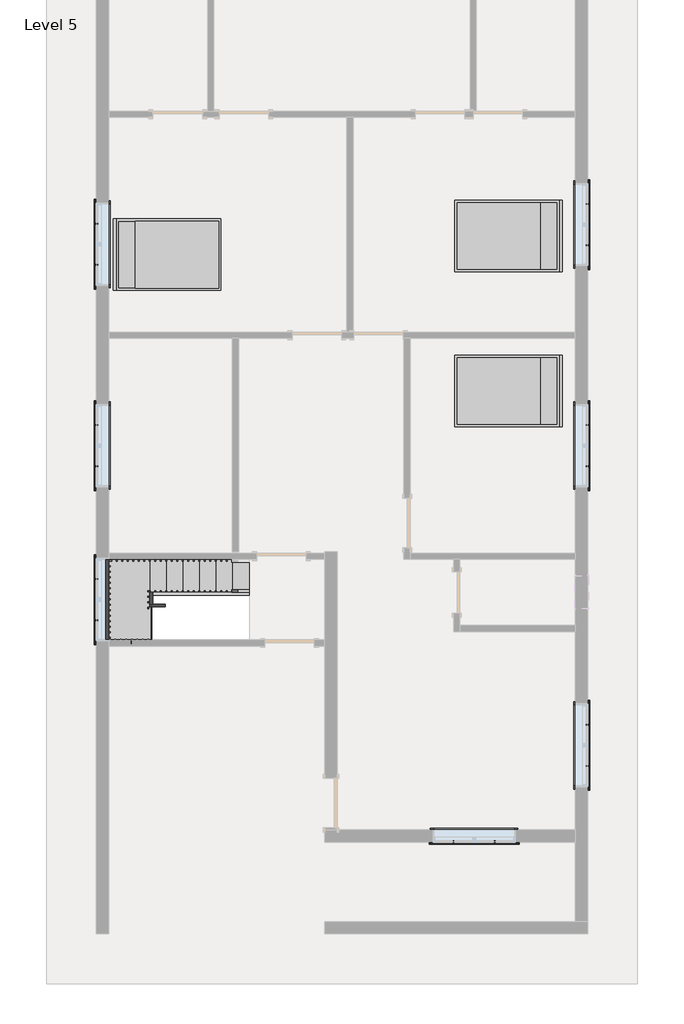
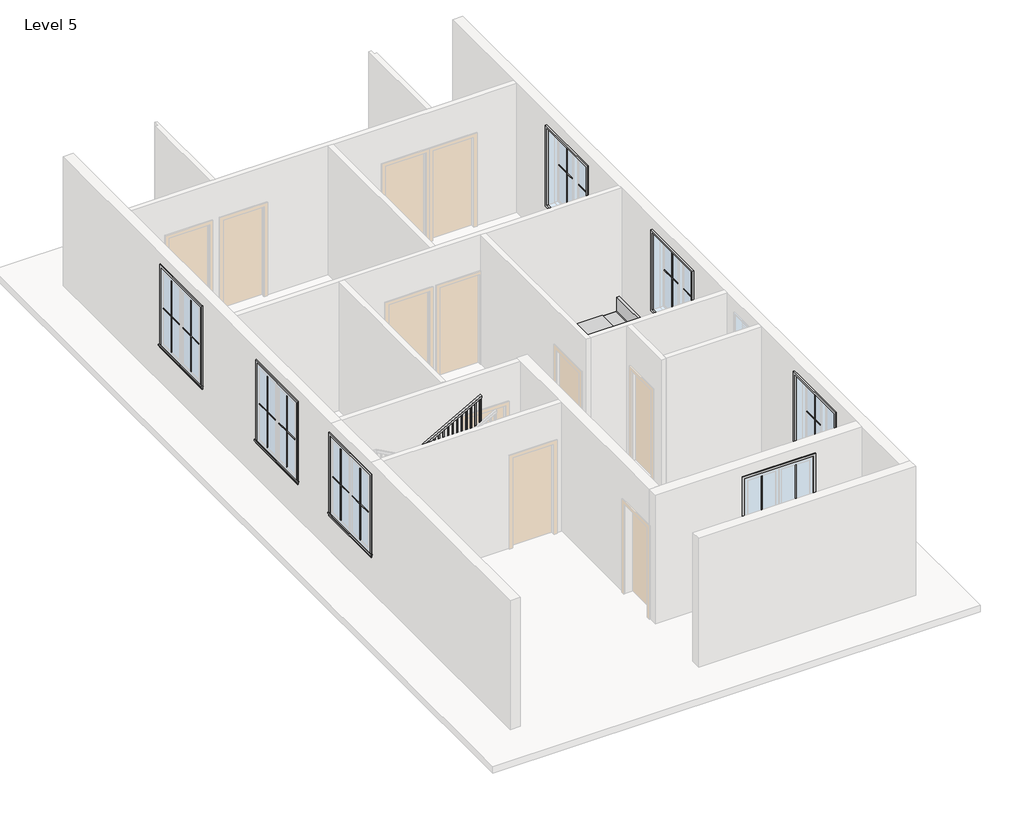
# One storey, part 3 of 3: 28 proxies, 6 members, 3 furniture elements, 1 railing, 1 stair flight.
"""IFC4 building model written with IfcOpenShell, lengths in millimetres."""

from ifc_helpers import new_model, si_unit, frame, origin, place, context, project, spatial, polyline, outline, extrude, faceted_brep, transform, mapped, element, save
from components import muntin_pattern_2x2_muntin_pattern_2x2_f6a80940, muntin_pattern_2x2_muntin_pattern_2x2_09b00a1c, trim_window_exterior_flat_with_sill_698ed857, trim_window_interior_flat_picture_frame_92551a5e, bed_17739_bed_17739_15c61121, stair_flight_98403923

model = new_model("IFC4")

# Units and contexts
model_context = context("Model", 3, world=origin())
ifc_project = project(units=[si_unit("LENGTHUNIT", "METRE", prefix="MILLI")], contexts=[model_context])

# Site, building, storey
site = spatial("IfcSite", under=ifc_project)
building = spatial("IfcBuilding", under=site)
storey = spatial("IfcBuildingStorey", under=building, Name="Level 5", Elevation=9601.2)

# Proxies
placement = place(None, origin())
muntin_pattern_2x2_muntin_pattern_2x2_shape = muntin_pattern_2x2_muntin_pattern_2x2_f6a80940(model_context)
element("IfcBuildingElementProxy", 1, Name="Muntin Pattern_2x2 : Muntin Pattern_2x2", ObjectType="Muntin Pattern_2x2 : Muntin Pattern_2x2", at=placement, inside=storey, context=model_context, shape_type="MappedRepresentation", body=[
    mapped(muntin_pattern_2x2_muntin_pattern_2x2_shape, transform((-5778.6870155, 3260.8309309, 10585.45), x_axis=(0.0, 1.0, 0.0), y_axis=(-1.0, 0.0, 0.0), z_axis=(0.0, 0.0, 1.0))),
])
element("IfcBuildingElementProxy", 2, Name="Muntin Pattern_2x2 : Muntin Pattern_2x2", ObjectType="Muntin Pattern_2x2 : Muntin Pattern_2x2", at=placement, inside=storey, context=model_context, shape_type="MappedRepresentation", body=[
    mapped(muntin_pattern_2x2_muntin_pattern_2x2_shape, transform((3270.0629845, 4381.6059309, 10585.45), x_axis=(0.0, -1.0, 0.0), y_axis=(1.0, 0.0, 0.0), z_axis=(0.0, 0.0, 1.0))),
])
element("IfcBuildingElementProxy", 3, Name="Muntin Pattern_2x2 : Muntin Pattern_2x2", ObjectType="Muntin Pattern_2x2 : Muntin Pattern_2x2", at=placement, inside=storey, context=model_context, shape_type="MappedRepresentation", body=[
    mapped(muntin_pattern_2x2_muntin_pattern_2x2_shape, transform((3270.0629845, 304.9059309, 10585.45), x_axis=(0.0, -1.0, 0.0), y_axis=(1.0, 0.0, 0.0), z_axis=(0.0, 0.0, 1.0))),
])
element("IfcBuildingElementProxy", 4, Name="Muntin Pattern_2x2 : Muntin Pattern_2x2", ObjectType="Muntin Pattern_2x2 : Muntin Pattern_2x2", at=placement, inside=storey, context=model_context, shape_type="MappedRepresentation", body=[
    mapped(muntin_pattern_2x2_muntin_pattern_2x2_shape, transform((3270.0629845, -5219.5940691, 10585.45), x_axis=(0.0, -1.0, 0.0), y_axis=(1.0, 0.0, 0.0), z_axis=(0.0, 0.0, 1.0))),
])
element("IfcBuildingElementProxy", 5, Name="Muntin Pattern_2x2 : Muntin Pattern_2x2", ObjectType="Muntin Pattern_2x2 : Muntin Pattern_2x2", at=placement, inside=storey, context=model_context, shape_type="MappedRepresentation", body=[
    mapped(muntin_pattern_2x2_muntin_pattern_2x2_shape, transform((1563.5004845, -7380.1815691, 10585.45), x_axis=(-1.0, 0.0, 0.0), y_axis=(0.0, -1.0, 0.0), z_axis=(0.0, 0.0, 1.0))),
])
element("IfcBuildingElementProxy", 6, Name="Muntin Pattern_2x2 : Muntin Pattern_2x2", ObjectType="Muntin Pattern_2x2 : Muntin Pattern_2x2", at=placement, inside=storey, context=model_context, shape_type="MappedRepresentation", body=[
    mapped(muntin_pattern_2x2_muntin_pattern_2x2_shape, transform((-5778.6870155, -3292.3690691, 10585.45), x_axis=(0.0, 1.0, 0.0), y_axis=(-1.0, 0.0, 0.0), z_axis=(0.0, 0.0, 1.0))),
])
element("IfcBuildingElementProxy", 7, Name="Muntin Pattern_2x2 : Muntin Pattern_2x2", ObjectType="Muntin Pattern_2x2 : Muntin Pattern_2x2", at=placement, inside=storey, context=model_context, shape_type="MappedRepresentation", body=[
    mapped(muntin_pattern_2x2_muntin_pattern_2x2_shape, transform((-5778.6870155, -453.9190691, 10585.45), x_axis=(0.0, 1.0, 0.0), y_axis=(-1.0, 0.0, 0.0), z_axis=(0.0, 0.0, 1.0))),
])
muntin_pattern_2x2_muntin_pattern_2x2_2_shape = muntin_pattern_2x2_muntin_pattern_2x2_09b00a1c(model_context)
element("IfcBuildingElementProxy", 8, Name="Muntin Pattern_2x2 : Muntin Pattern_2x2", ObjectType="Muntin Pattern_2x2 : Muntin Pattern_2x2", at=placement, inside=storey, context=model_context, shape_type="MappedRepresentation", body=[
    mapped(muntin_pattern_2x2_muntin_pattern_2x2_2_shape, transform((-5778.6870155, 4019.6559309, 10585.45), x_axis=(0.0, -1.0, 0.0), y_axis=(1.0, 0.0, 0.0), z_axis=(0.0, 0.0, 1.0))),
])
element("IfcBuildingElementProxy", 9, Name="Muntin Pattern_2x2 : Muntin Pattern_2x2", ObjectType="Muntin Pattern_2x2 : Muntin Pattern_2x2", at=placement, inside=storey, context=model_context, shape_type="MappedRepresentation", body=[
    mapped(muntin_pattern_2x2_muntin_pattern_2x2_2_shape, transform((3270.0629845, 3622.7809309, 10585.45), x_axis=(0.0, 1.0, 0.0), y_axis=(-1.0, 0.0, 0.0), z_axis=(0.0, 0.0, 1.0))),
])
element("IfcBuildingElementProxy", 10, Name="Muntin Pattern_2x2 : Muntin Pattern_2x2", ObjectType="Muntin Pattern_2x2 : Muntin Pattern_2x2", at=placement, inside=storey, context=model_context, shape_type="MappedRepresentation", body=[
    mapped(muntin_pattern_2x2_muntin_pattern_2x2_2_shape, transform((3270.0629845, -453.9190691, 10585.45), x_axis=(0.0, 1.0, 0.0), y_axis=(-1.0, 0.0, 0.0), z_axis=(0.0, 0.0, 1.0))),
])
element("IfcBuildingElementProxy", 11, Name="Muntin Pattern_2x2 : Muntin Pattern_2x2", ObjectType="Muntin Pattern_2x2 : Muntin Pattern_2x2", at=placement, inside=storey, context=model_context, shape_type="MappedRepresentation", body=[
    mapped(muntin_pattern_2x2_muntin_pattern_2x2_2_shape, transform((3270.0629845, -5978.4190691, 10585.45), x_axis=(0.0, 1.0, 0.0), y_axis=(-1.0, 0.0, 0.0), z_axis=(0.0, 0.0, 1.0))),
])
element("IfcBuildingElementProxy", 12, Name="Muntin Pattern_2x2 : Muntin Pattern_2x2", ObjectType="Muntin Pattern_2x2 : Muntin Pattern_2x2", at=placement, inside=storey, context=model_context, shape_type="MappedRepresentation", body=[
    mapped(muntin_pattern_2x2_muntin_pattern_2x2_2_shape, transform((804.6754845, -7380.1815691, 10585.45), x_axis=(1.0, 0.0, 0.0), y_axis=(0.0, 1.0, 0.0), z_axis=(0.0, 0.0, 1.0))),
])
element("IfcBuildingElementProxy", 13, Name="Muntin Pattern_2x2 : Muntin Pattern_2x2", ObjectType="Muntin Pattern_2x2 : Muntin Pattern_2x2", at=placement, inside=storey, context=model_context, shape_type="MappedRepresentation", body=[
    mapped(muntin_pattern_2x2_muntin_pattern_2x2_2_shape, transform((-5778.6870155, -2533.5440691, 10585.45), x_axis=(0.0, -1.0, 0.0), y_axis=(1.0, 0.0, 0.0), z_axis=(0.0, 0.0, 1.0))),
])
element("IfcBuildingElementProxy", 14, Name="Muntin Pattern_2x2 : Muntin Pattern_2x2", ObjectType="Muntin Pattern_2x2 : Muntin Pattern_2x2", at=placement, inside=storey, context=model_context, shape_type="MappedRepresentation", body=[
    mapped(muntin_pattern_2x2_muntin_pattern_2x2_2_shape, transform((-5778.6870155, 304.9059309, 10585.45), x_axis=(0.0, -1.0, 0.0), y_axis=(1.0, 0.0, 0.0), z_axis=(0.0, 0.0, 1.0))),
])
trim_window_exterior_flat_with_sill_shape = trim_window_exterior_flat_with_sill_698ed857(model_context)
element("IfcBuildingElementProxy", 15, Name="Trim-Window-Exterior-Flat : with Sill", ObjectType="Trim-Window-Exterior-Flat : with Sill", at=placement, inside=storey, context=model_context, shape_type="MappedRepresentation", body=[
    mapped(trim_window_exterior_flat_with_sill_shape, transform((-5788.2120155, 3640.2434309, 12344.4), x_axis=(0.0, -1.0, 0.0), y_axis=(0.0, 0.0, 1.0), z_axis=(-1.0, 0.0, 0.0))),
])
element("IfcBuildingElementProxy", 16, Name="Trim-Window-Exterior-Flat : with Sill", ObjectType="Trim-Window-Exterior-Flat : with Sill", at=placement, inside=storey, context=model_context, shape_type="MappedRepresentation", body=[
    mapped(trim_window_exterior_flat_with_sill_shape, transform((3279.5879845, 4002.1934309, 12344.4), x_axis=(0.0, 1.0, 0.0), y_axis=(0.0, 0.0, 1.0), z_axis=(1.0, 0.0, 0.0))),
])
element("IfcBuildingElementProxy", 17, Name="Trim-Window-Exterior-Flat : with Sill", ObjectType="Trim-Window-Exterior-Flat : with Sill", at=placement, inside=storey, context=model_context, shape_type="MappedRepresentation", body=[
    mapped(trim_window_exterior_flat_with_sill_shape, transform((3279.5879845, -74.5065691, 12344.4), x_axis=(0.0, 1.0, 0.0), y_axis=(0.0, 0.0, 1.0), z_axis=(1.0, 0.0, 0.0))),
])
element("IfcBuildingElementProxy", 18, Name="Trim-Window-Exterior-Flat : with Sill", ObjectType="Trim-Window-Exterior-Flat : with Sill", at=placement, inside=storey, context=model_context, shape_type="MappedRepresentation", body=[
    mapped(trim_window_exterior_flat_with_sill_shape, transform((3279.5879845, -5599.0065691, 12344.4), x_axis=(0.0, 1.0, 0.0), y_axis=(0.0, 0.0, 1.0), z_axis=(1.0, 0.0, 0.0))),
])
element("IfcBuildingElementProxy", 19, Name="Trim-Window-Exterior-Flat : with Sill", ObjectType="Trim-Window-Exterior-Flat : with Sill", at=placement, inside=storey, context=model_context, shape_type="MappedRepresentation", body=[
    mapped(trim_window_exterior_flat_with_sill_shape, transform((1184.0879845, -7389.7065691, 12344.4), x_axis=(1.0, 0.0, 0.0), y_axis=(0.0, 0.0, 1.0), z_axis=(0.0, -1.0, 0.0))),
])
element("IfcBuildingElementProxy", 20, Name="Trim-Window-Exterior-Flat : with Sill", ObjectType="Trim-Window-Exterior-Flat : with Sill", at=placement, inside=storey, context=model_context, shape_type="MappedRepresentation", body=[
    mapped(trim_window_exterior_flat_with_sill_shape, transform((-5788.2120155, -2912.9565691, 12344.4), x_axis=(0.0, -1.0, 0.0), y_axis=(0.0, 0.0, 1.0), z_axis=(-1.0, 0.0, 0.0))),
])
element("IfcBuildingElementProxy", 21, Name="Trim-Window-Exterior-Flat : with Sill", ObjectType="Trim-Window-Exterior-Flat : with Sill", at=placement, inside=storey, context=model_context, shape_type="MappedRepresentation", body=[
    mapped(trim_window_exterior_flat_with_sill_shape, transform((-5788.2120155, -74.5065691, 12344.4), x_axis=(0.0, -1.0, 0.0), y_axis=(0.0, 0.0, 1.0), z_axis=(-1.0, 0.0, 0.0))),
])
trim_window_interior_flat_picture_frame_shape = trim_window_interior_flat_picture_frame_92551a5e(model_context)
element("IfcBuildingElementProxy", 22, Name="Trim-Window-Interior-Flat : Picture Frame", ObjectType="Trim-Window-Interior-Flat : Picture Frame", at=placement, inside=storey, context=model_context, shape_type="MappedRepresentation", body=[
    mapped(trim_window_interior_flat_picture_frame_shape, transform((-5559.6120155, 3640.2434309, 12344.4), x_axis=(0.0, 1.0, 0.0), y_axis=(0.0, 0.0, 1.0), z_axis=(1.0, 0.0, 0.0))),
])
element("IfcBuildingElementProxy", 23, Name="Trim-Window-Interior-Flat : Picture Frame", ObjectType="Trim-Window-Interior-Flat : Picture Frame", at=placement, inside=storey, context=model_context, shape_type="MappedRepresentation", body=[
    mapped(trim_window_interior_flat_picture_frame_shape, transform((3050.9879845, 4002.1934309, 12344.4), x_axis=(0.0, -1.0, 0.0), y_axis=(0.0, 0.0, 1.0), z_axis=(-1.0, 0.0, 0.0))),
])
element("IfcBuildingElementProxy", 24, Name="Trim-Window-Interior-Flat : Picture Frame", ObjectType="Trim-Window-Interior-Flat : Picture Frame", at=placement, inside=storey, context=model_context, shape_type="MappedRepresentation", body=[
    mapped(trim_window_interior_flat_picture_frame_shape, transform((3050.9879845, -74.5065691, 12344.4), x_axis=(0.0, -1.0, 0.0), y_axis=(0.0, 0.0, 1.0), z_axis=(-1.0, 0.0, 0.0))),
])
element("IfcBuildingElementProxy", 25, Name="Trim-Window-Interior-Flat : Picture Frame", ObjectType="Trim-Window-Interior-Flat : Picture Frame", at=placement, inside=storey, context=model_context, shape_type="MappedRepresentation", body=[
    mapped(trim_window_interior_flat_picture_frame_shape, transform((3050.9879845, -5599.0065691, 12344.4), x_axis=(0.0, -1.0, 0.0), y_axis=(0.0, 0.0, 1.0), z_axis=(-1.0, 0.0, 0.0))),
])
element("IfcBuildingElementProxy", 26, Name="Trim-Window-Interior-Flat : Picture Frame", ObjectType="Trim-Window-Interior-Flat : Picture Frame", at=placement, inside=storey, context=model_context, shape_type="MappedRepresentation", body=[
    mapped(trim_window_interior_flat_picture_frame_shape, transform((1184.0879845, -7161.1065691, 12344.4), x_axis=(-1.0, 0.0, 0.0), y_axis=(0.0, 0.0, 1.0), z_axis=(0.0, 1.0, 0.0))),
])
element("IfcBuildingElementProxy", 27, Name="Trim-Window-Interior-Flat : Picture Frame", ObjectType="Trim-Window-Interior-Flat : Picture Frame", at=placement, inside=storey, context=model_context, shape_type="MappedRepresentation", body=[
    mapped(trim_window_interior_flat_picture_frame_shape, transform((-5559.6120155, -2912.9565691, 12344.4), x_axis=(0.0, 1.0, 0.0), y_axis=(0.0, 0.0, 1.0), z_axis=(1.0, 0.0, 0.0))),
])
element("IfcBuildingElementProxy", 28, Name="Trim-Window-Interior-Flat : Picture Frame", ObjectType="Trim-Window-Interior-Flat : Picture Frame", at=placement, inside=storey, context=model_context, shape_type="MappedRepresentation", body=[
    mapped(trim_window_interior_flat_picture_frame_shape, transform((-5559.6120155, -74.5065691, 12344.4), x_axis=(0.0, 1.0, 0.0), y_axis=(0.0, 0.0, 1.0), z_axis=(1.0, 0.0, 0.0))),
])

# Furniture
bed_17739_bed_17739_shape = bed_17739_bed_17739_15c61121(model_context)
element("IfcFurniture", 29, ObjectType="Bed_17739 : Bed_17739", at=placement, inside=storey, context=model_context, shape_type="MappedRepresentation", body=[
    mapped(bed_17739_bed_17739_shape, transform((-4454.7120155, 3449.7434309, 9601.2), x_axis=(0.0, 1.0, 0.0), y_axis=(-1.0, 0.0, 0.0), z_axis=(0.0, 0.0, 1.0))),
])
element("IfcFurniture", 30, ObjectType="Bed_17739 : Bed_17739", at=placement, inside=storey, context=model_context, shape_type="MappedRepresentation", body=[
    mapped(bed_17739_bed_17739_shape, transform((1793.6879845, 3792.6434309, 9601.2), x_axis=(0.0, -1.0, 0.0), y_axis=(1.0, 0.0, 0.0), z_axis=(0.0, 0.0, 1.0))),
])
element("IfcFurniture", 31, ObjectType="Bed_17739 : Bed_17739", at=placement, inside=storey, context=model_context, shape_type="MappedRepresentation", body=[
    mapped(bed_17739_bed_17739_shape, transform((1793.6879845, 935.1434309, 9601.2), x_axis=(0.0, -1.0, 0.0), y_axis=(1.0, 0.0, 0.0), z_axis=(0.0, 0.0, 1.0))),
])

# Members
element("IfcMember", 32, ObjectType="Stringer - 2\" Width", at=placement, inside=storey, context=model_context, shape_type="SweptSolid", body=[
    extrude(outline(polyline([(9601.2, -2968.8120155), (9808.7983948, -2968.8120155), (10796.5761726, -4746.8120155), (10447.8974984, -4746.8120155), (9601.2, -3222.7565183), (9601.2, -2968.8120155)])), frame((0.0, -2830.4065691, 0.0), z_axis=(0.0, 1.0, 0.0), x_axis=(0.0, 0.0, 1.0)), (0.0, 0.0, 1.0), 50.8),
])
element("IfcMember", 33, ObjectType="Stringer - 2\" Width", at=placement, inside=storey, context=model_context, shape_type="SweptSolid", body=[
    extrude(outline(polyline([(-4797.6120155, -2779.6065691), (-4746.8120155, -2779.6065691), (-4746.8120155, -2995.5065691), (-4797.6120155, -2995.5065691), (-4797.6120155, -2779.6065691)])), frame((0.0, 0.0, 10557.9333333), z_axis=(0.0, 0.0, 1.0), x_axis=(1.0, 0.0, 0.0)), (0.0, 0.0, 1.0), 304.8),
])
element("IfcMember", 34, ObjectType="Stringer - 2\" Width", at=placement, inside=storey, context=model_context, shape_type="SweptSolid", body=[
    extrude(outline(polyline([(10994.1317281, -4797.6120155), (10645.453054, -4797.6120155), (11661.453054, -2968.8120155), (12010.1317281, -2968.8120155), (10994.1317281, -4797.6120155)])), frame((0.0, -3046.3065691, 0.0), z_axis=(0.0, 1.0, 0.0), x_axis=(0.0, 0.0, 1.0)), (0.0, 0.0, 1.0), 50.8),
])
element("IfcMember", 35, ObjectType="Stringer - 2\" Width", at=placement, inside=storey, context=model_context, shape_type="SweptSolid", body=[
    extrude(outline(polyline([(9601.2, -2968.8120155), (9808.7983948, -2968.8120155), (10862.7333333, -4865.8949049), (10862.7333333, -5493.5165183), (9601.2, -3222.7565183), (9601.2, -2968.8120155)])), frame((0.0, -2170.0065691, 0.0), z_axis=(0.0, 1.0, 0.0), x_axis=(0.0, 0.0, 1.0)), (0.0, 0.0, 1.0), 50.8),
])
element("IfcMember", 36, ObjectType="Stringer - 2\" Width", at=placement, inside=storey, context=model_context, shape_type="SweptSolid", body=[
    extrude(outline(polyline([(-5610.4120155, -2119.2065691), (-5559.6120155, -2119.2065691), (-5559.6120155, -3674.9565691), (-5610.4120155, -3674.9565691), (-5610.4120155, -2119.2065691)])), frame((0.0, 0.0, 10557.9333333), z_axis=(0.0, 0.0, 1.0), x_axis=(1.0, 0.0, 0.0)), (0.0, 0.0, 1.0), 304.8),
])
element("IfcMember", 37, ObjectType="Stringer - 2\" Width", at=placement, inside=storey, context=model_context, shape_type="SweptSolid", body=[
    extrude(outline(polyline([(10557.9333333, -4955.1475127), (11661.453054, -2968.8120155), (12010.1317281, -2968.8120155), (10557.9333333, -5582.7691261), (10557.9333333, -4955.1475127)])), frame((0.0, -3725.7565691, 0.0), z_axis=(0.0, 1.0, 0.0), x_axis=(0.0, 0.0, 1.0)), (0.0, 0.0, 1.0), 50.8),
])

# Railing
element("IfcRailing", 38, ObjectType="Handrail - Rectangular", at=placement, inside=storey, context=model_context, shape_type="SolidModel", body=[
    faceted_brep([(-2968.8120155, -2779.6065691, 10684.9333333), (-2968.8120155, -2779.6065691, 10626.820221), (-2968.8120155, -2728.8065691, 10626.820221), (-2968.8120155, -2728.8065691, 10684.9333333), (-4721.4120155, -2779.6065691, 11658.6), (-4772.2120155, -2779.6065691, 11628.7091099), (-4772.2120155, -2728.8065691, 11628.7091099), (-4721.4120155, -2728.8065691, 11658.6), (-4721.4120155, -2779.6065691, 11700.9333333), (-4772.2120155, -2779.6065691, 11650.1333333), (-4772.2120155, -2728.8065691, 11650.1333333), (-4721.4120155, -2728.8065691, 11700.9333333), (-4797.6120155, -2779.6065691, 11700.9333333), (-4797.6120155, -2779.6065691, 11650.1333333), (-4848.4120155, -2728.8065691, 11650.1333333), (-4848.4120155, -2728.8065691, 11700.9333333), (-4797.6120155, -2855.8065691, 11700.9333333), (-4797.6120155, -2855.8065691, 11650.1333333), (-4848.4120155, -2855.8065691, 11650.1333333), (-4848.4120155, -2855.8065691, 11700.9333333), (-4797.6120155, -2970.1065691, 11700.9333333), (-4797.6120155, -3020.9065691, 11650.1333333), (-4848.4120155, -3020.9065691, 11650.1333333), (-4848.4120155, -2970.1065691, 11700.9333333), (-4797.6120155, -2970.1065691, 11912.6), (-4797.6120155, -3020.9065691, 11861.8), (-4848.4120155, -3020.9065691, 11861.8), (-4848.4120155, -2970.1065691, 11912.6), (-4797.6120155, -3046.3065691, 11912.6), (-4797.6120155, -3046.3065691, 11861.8), (-4848.4120155, -3097.1065691, 11861.8), (-4848.4120155, -3097.1065691, 11912.6), (-4721.4120155, -3046.3065691, 11912.6), (-4708.2484132, -3046.3065691, 11861.8), (-4708.2484132, -3097.1065691, 11861.8), (-4721.4120155, -3097.1065691, 11912.6), (-2968.8120155, -3046.3065691, 12886.2666667), (-2968.8120155, -3097.1065691, 12886.2666667), (-2968.8120155, -3097.1065691, 12828.1535543), (-2968.8120155, -3046.3065691, 12828.1535543)], [[[0, 1, 2, 3]], [[1, 0, 4, 5]], [[2, 1, 5, 6]], [[3, 2, 6, 7]], [[0, 3, 7, 4]], [[5, 4, 8, 9]], [[6, 5, 9, 10]], [[7, 6, 10, 11]], [[4, 7, 11, 8]], [[9, 8, 12, 13]], [[10, 9, 13, 14]], [[11, 10, 14, 15]], [[8, 11, 15, 12]], [[13, 12, 16, 17]], [[14, 13, 17, 18]], [[15, 14, 18, 19]], [[12, 15, 19, 16]], [[17, 16, 20, 21]], [[18, 17, 21, 22]], [[19, 18, 22, 23]], [[16, 19, 23, 20]], [[21, 20, 24, 25]], [[22, 21, 25, 26]], [[23, 22, 26, 27]], [[20, 23, 27, 24]], [[25, 24, 28, 29]], [[26, 25, 29, 30]], [[27, 26, 30, 31]], [[24, 27, 31, 28]], [[29, 28, 32, 33]], [[30, 29, 33, 34]], [[31, 30, 34, 35]], [[28, 31, 35, 32]], [[36, 37, 38, 39]], [[33, 32, 36, 39]], [[34, 33, 39, 38]], [[35, 34, 38, 37]], [[32, 35, 37, 36]]]),
    extrude(outline(polyline([(12808.7507765, -3003.7370155), (11802.5333333, -3003.7370155), (11802.5333333, -2984.6870155), (12819.3341099, -2984.6870155), (12808.7507765, -3003.7370155)])), frame((0.0, -3081.2315691, 0.0), z_axis=(0.0, 1.0, 0.0), x_axis=(0.0, 0.0, 1.0)), (0.0, 0.0, 1.0), 19.05),
    extrude(outline(polyline([(12752.3063321, -3105.3370155), (11802.5333333, -3105.3370155), (11802.5333333, -3086.2870155), (12762.8896654, -3086.2870155), (12752.3063321, -3105.3370155)])), frame((0.0, -3081.2315691, 0.0), z_axis=(0.0, 1.0, 0.0), x_axis=(0.0, 0.0, 1.0)), (0.0, 0.0, 1.0), 19.05),
    extrude(outline(polyline([(12695.8618876, -3206.9370155), (11802.5333333, -3206.9370155), (11802.5333333, -3187.8870155), (12706.445221, -3187.8870155), (12695.8618876, -3206.9370155)])), frame((0.0, -3081.2315691, 0.0), z_axis=(0.0, 1.0, 0.0), x_axis=(0.0, 0.0, 1.0)), (0.0, 0.0, 1.0), 19.05),
    extrude(outline(polyline([(12639.4174432, -3308.5370155), (11633.2, -3308.5370155), (11633.2, -3289.4870155), (12650.0007765, -3289.4870155), (12639.4174432, -3308.5370155)])), frame((0.0, -3081.2315691, 0.0), z_axis=(0.0, 1.0, 0.0), x_axis=(0.0, 0.0, 1.0)), (0.0, 0.0, 1.0), 19.05),
    extrude(outline(polyline([(12582.9729988, -3410.1370155), (11633.2, -3410.1370155), (11633.2, -3391.0870155), (12593.5563321, -3391.0870155), (12582.9729988, -3410.1370155)])), frame((0.0, -3081.2315691, 0.0), z_axis=(0.0, 1.0, 0.0), x_axis=(0.0, 0.0, 1.0)), (0.0, 0.0, 1.0), 19.05),
    extrude(outline(polyline([(12526.5285543, -3511.7370155), (11633.2, -3511.7370155), (11633.2, -3492.6870155), (12537.1118876, -3492.6870155), (12526.5285543, -3511.7370155)])), frame((0.0, -3081.2315691, 0.0), z_axis=(0.0, 1.0, 0.0), x_axis=(0.0, 0.0, 1.0)), (0.0, 0.0, 1.0), 19.05),
    extrude(outline(polyline([(12470.0841099, -3613.3370155), (11463.8666667, -3613.3370155), (11463.8666667, -3594.2870155), (12480.6674432, -3594.2870155), (12470.0841099, -3613.3370155)])), frame((0.0, -3081.2315691, 0.0), z_axis=(0.0, 1.0, 0.0), x_axis=(0.0, 0.0, 1.0)), (0.0, 0.0, 1.0), 19.05),
    extrude(outline(polyline([(12413.6396654, -3714.9370155), (11463.8666667, -3714.9370155), (11463.8666667, -3695.8870155), (12424.2229988, -3695.8870155), (12413.6396654, -3714.9370155)])), frame((0.0, -3081.2315691, 0.0), z_axis=(0.0, 1.0, 0.0), x_axis=(0.0, 0.0, 1.0)), (0.0, 0.0, 1.0), 19.05),
    extrude(outline(polyline([(12357.195221, -3816.5370155), (11463.8666667, -3816.5370155), (11463.8666667, -3797.4870155), (12367.7785543, -3797.4870155), (12357.195221, -3816.5370155)])), frame((0.0, -3081.2315691, 0.0), z_axis=(0.0, 1.0, 0.0), x_axis=(0.0, 0.0, 1.0)), (0.0, 0.0, 1.0), 19.05),
    extrude(outline(polyline([(12300.7507765, -3918.1370155), (11294.5333333, -3918.1370155), (11294.5333333, -3899.0870155), (12311.3341099, -3899.0870155), (12300.7507765, -3918.1370155)])), frame((0.0, -3081.2315691, 0.0), z_axis=(0.0, 1.0, 0.0), x_axis=(0.0, 0.0, 1.0)), (0.0, 0.0, 1.0), 19.05),
    extrude(outline(polyline([(12244.3063321, -4019.7370155), (11294.5333333, -4019.7370155), (11294.5333333, -4000.6870155), (12254.8896654, -4000.6870155), (12244.3063321, -4019.7370155)])), frame((0.0, -3081.2315691, 0.0), z_axis=(0.0, 1.0, 0.0), x_axis=(0.0, 0.0, 1.0)), (0.0, 0.0, 1.0), 19.05),
    extrude(outline(polyline([(12187.8618876, -4121.3370155), (11294.5333333, -4121.3370155), (11294.5333333, -4102.2870155), (12198.445221, -4102.2870155), (12187.8618876, -4121.3370155)])), frame((0.0, -3081.2315691, 0.0), z_axis=(0.0, 1.0, 0.0), x_axis=(0.0, 0.0, 1.0)), (0.0, 0.0, 1.0), 19.05),
    extrude(outline(polyline([(12131.4174432, -4222.9370155), (11125.2, -4222.9370155), (11125.2, -4203.8870155), (12142.0007765, -4203.8870155), (12131.4174432, -4222.9370155)])), frame((0.0, -3081.2315691, 0.0), z_axis=(0.0, 1.0, 0.0), x_axis=(0.0, 0.0, 1.0)), (0.0, 0.0, 1.0), 19.05),
    extrude(outline(polyline([(12074.9729988, -4324.5370155), (11125.2, -4324.5370155), (11125.2, -4305.4870155), (12085.5563321, -4305.4870155), (12074.9729988, -4324.5370155)])), frame((0.0, -3081.2315691, 0.0), z_axis=(0.0, 1.0, 0.0), x_axis=(0.0, 0.0, 1.0)), (0.0, 0.0, 1.0), 19.05),
    extrude(outline(polyline([(12018.5285543, -4426.1370155), (11125.2, -4426.1370155), (11125.2, -4407.0870155), (12029.1118876, -4407.0870155), (12018.5285543, -4426.1370155)])), frame((0.0, -3081.2315691, 0.0), z_axis=(0.0, 1.0, 0.0), x_axis=(0.0, 0.0, 1.0)), (0.0, 0.0, 1.0), 19.05),
    extrude(outline(polyline([(11962.0841099, -4527.7370155), (10955.8666667, -4527.7370155), (10955.8666667, -4508.6870155), (11972.6674432, -4508.6870155), (11962.0841099, -4527.7370155)])), frame((0.0, -3081.2315691, 0.0), z_axis=(0.0, 1.0, 0.0), x_axis=(0.0, 0.0, 1.0)), (0.0, 0.0, 1.0), 19.05),
    extrude(outline(polyline([(11905.6396654, -4629.3370155), (10955.8666667, -4629.3370155), (10955.8666667, -4610.2870155), (11916.2229988, -4610.2870155), (11905.6396654, -4629.3370155)])), frame((0.0, -3081.2315691, 0.0), z_axis=(0.0, 1.0, 0.0), x_axis=(0.0, 0.0, 1.0)), (0.0, 0.0, 1.0), 19.05),
    extrude(outline(polyline([(11849.195221, -4730.9370155), (10955.8666667, -4730.9370155), (10955.8666667, -4711.8870155), (11859.7785543, -4711.8870155), (11849.195221, -4730.9370155)])), frame((0.0, -3081.2315691, 0.0), z_axis=(0.0, 1.0, 0.0), x_axis=(0.0, 0.0, 1.0)), (0.0, 0.0, 1.0), 19.05),
    extrude(outline(polyline([(-4813.4870155, -3049.4815691), (-4813.4870155, -3068.5315691), (-4832.5370155, -3068.5315691), (-4832.5370155, -3049.4815691), (-4813.4870155, -3049.4815691)])), frame((0.0, 0.0, 10786.5333333), z_axis=(0.0, 0.0, 1.0), x_axis=(1.0, 0.0, 0.0)), (0.0, 0.0, 1.0), 1075.2666667),
    extrude(outline(polyline([(-4813.4870155, -2947.8815691), (-4813.4870155, -2966.9315691), (-4832.5370155, -2966.9315691), (-4832.5370155, -2947.8815691), (-4813.4870155, -2947.8815691)])), frame((0.0, 0.0, 10786.5333333), z_axis=(0.0, 0.0, 1.0), x_axis=(1.0, 0.0, 0.0)), (0.0, 0.0, 1.0), 863.6),
    extrude(outline(polyline([(-4813.4870155, -2846.2815691), (-4813.4870155, -2865.3315691), (-4832.5370155, -2865.3315691), (-4832.5370155, -2846.2815691), (-4813.4870155, -2846.2815691)])), frame((0.0, 0.0, 10786.5333333), z_axis=(0.0, 0.0, 1.0), x_axis=(1.0, 0.0, 0.0)), (0.0, 0.0, 1.0), 863.6),
    extrude(outline(polyline([(-4788.0870155, -2763.7315691), (-4807.1370155, -2763.7315691), (-4807.1370155, -2744.6815691), (-4788.0870155, -2744.6815691), (-4788.0870155, -2763.7315691)])), frame((0.0, 0.0, 10786.5333333), z_axis=(0.0, 0.0, 1.0), x_axis=(1.0, 0.0, 0.0)), (0.0, 0.0, 1.0), 863.6),
    extrude(outline(polyline([(11591.6674432, -4705.5370155), (10617.2, -4705.5370155), (10617.2, -4686.4870155), (11581.0841099, -4686.4870155), (11591.6674432, -4705.5370155)])), frame((0.0, -2763.7315691, 0.0), z_axis=(0.0, 1.0, 0.0), x_axis=(0.0, 0.0, 1.0)), (0.0, 0.0, 1.0), 19.05),
    extrude(outline(polyline([(11535.2229988, -4603.9370155), (10617.2, -4603.9370155), (10617.2, -4584.8870155), (11524.6396654, -4584.8870155), (11535.2229988, -4603.9370155)])), frame((0.0, -2763.7315691, 0.0), z_axis=(0.0, 1.0, 0.0), x_axis=(0.0, 0.0, 1.0)), (0.0, 0.0, 1.0), 19.05),
    extrude(outline(polyline([(11478.7785543, -4502.3370155), (10617.2, -4502.3370155), (10617.2, -4483.2870155), (11468.195221, -4483.2870155), (11478.7785543, -4502.3370155)])), frame((0.0, -2763.7315691, 0.0), z_axis=(0.0, 1.0, 0.0), x_axis=(0.0, 0.0, 1.0)), (0.0, 0.0, 1.0), 19.05),
    extrude(outline(polyline([(11422.3341099, -4400.7370155), (10447.8666667, -4400.7370155), (10447.8666667, -4381.6870155), (11411.7507765, -4381.6870155), (11422.3341099, -4400.7370155)])), frame((0.0, -2763.7315691, 0.0), z_axis=(0.0, 1.0, 0.0), x_axis=(0.0, 0.0, 1.0)), (0.0, 0.0, 1.0), 19.05),
    extrude(outline(polyline([(11365.8896654, -4299.1370155), (10447.8666667, -4299.1370155), (10447.8666667, -4280.0870155), (11355.3063321, -4280.0870155), (11365.8896654, -4299.1370155)])), frame((0.0, -2763.7315691, 0.0), z_axis=(0.0, 1.0, 0.0), x_axis=(0.0, 0.0, 1.0)), (0.0, 0.0, 1.0), 19.05),
    extrude(outline(polyline([(11309.445221, -4197.5370155), (10447.8666667, -4197.5370155), (10447.8666667, -4178.4870155), (11298.8618876, -4178.4870155), (11309.445221, -4197.5370155)])), frame((0.0, -2763.7315691, 0.0), z_axis=(0.0, 1.0, 0.0), x_axis=(0.0, 0.0, 1.0)), (0.0, 0.0, 1.0), 19.05),
    extrude(outline(polyline([(11253.0007765, -4095.9370155), (10278.5333333, -4095.9370155), (10278.5333333, -4076.8870155), (11242.4174432, -4076.8870155), (11253.0007765, -4095.9370155)])), frame((0.0, -2763.7315691, 0.0), z_axis=(0.0, 1.0, 0.0), x_axis=(0.0, 0.0, 1.0)), (0.0, 0.0, 1.0), 19.05),
    extrude(outline(polyline([(11196.5563321, -3994.3370155), (10278.5333333, -3994.3370155), (10278.5333333, -3975.2870155), (11185.9729988, -3975.2870155), (11196.5563321, -3994.3370155)])), frame((0.0, -2763.7315691, 0.0), z_axis=(0.0, 1.0, 0.0), x_axis=(0.0, 0.0, 1.0)), (0.0, 0.0, 1.0), 19.05),
    extrude(outline(polyline([(11140.1118876, -3892.7370155), (10278.5333333, -3892.7370155), (10278.5333333, -3873.6870155), (11129.5285543, -3873.6870155), (11140.1118876, -3892.7370155)])), frame((0.0, -2763.7315691, 0.0), z_axis=(0.0, 1.0, 0.0), x_axis=(0.0, 0.0, 1.0)), (0.0, 0.0, 1.0), 19.05),
    extrude(outline(polyline([(11083.6674432, -3791.1370155), (10109.2, -3791.1370155), (10109.2, -3772.0870155), (11073.0841099, -3772.0870155), (11083.6674432, -3791.1370155)])), frame((0.0, -2763.7315691, 0.0), z_axis=(0.0, 1.0, 0.0), x_axis=(0.0, 0.0, 1.0)), (0.0, 0.0, 1.0), 19.05),
    extrude(outline(polyline([(11027.2229988, -3689.5370155), (10109.2, -3689.5370155), (10109.2, -3670.4870155), (11016.6396654, -3670.4870155), (11027.2229988, -3689.5370155)])), frame((0.0, -2763.7315691, 0.0), z_axis=(0.0, 1.0, 0.0), x_axis=(0.0, 0.0, 1.0)), (0.0, 0.0, 1.0), 19.05),
    extrude(outline(polyline([(10970.7785543, -3587.9370155), (10109.2, -3587.9370155), (10109.2, -3568.8870155), (10960.195221, -3568.8870155), (10970.7785543, -3587.9370155)])), frame((0.0, -2763.7315691, 0.0), z_axis=(0.0, 1.0, 0.0), x_axis=(0.0, 0.0, 1.0)), (0.0, 0.0, 1.0), 19.05),
    extrude(outline(polyline([(10914.3341099, -3486.3370155), (9939.8666667, -3486.3370155), (9939.8666667, -3467.2870155), (10903.7507765, -3467.2870155), (10914.3341099, -3486.3370155)])), frame((0.0, -2763.7315691, 0.0), z_axis=(0.0, 1.0, 0.0), x_axis=(0.0, 0.0, 1.0)), (0.0, 0.0, 1.0), 19.05),
    extrude(outline(polyline([(10857.8896654, -3384.7370155), (9939.8666667, -3384.7370155), (9939.8666667, -3365.6870155), (10847.3063321, -3365.6870155), (10857.8896654, -3384.7370155)])), frame((0.0, -2763.7315691, 0.0), z_axis=(0.0, 1.0, 0.0), x_axis=(0.0, 0.0, 1.0)), (0.0, 0.0, 1.0), 19.05),
    extrude(outline(polyline([(10801.445221, -3283.1370155), (9939.8666667, -3283.1370155), (9939.8666667, -3264.0870155), (10790.8618876, -3264.0870155), (10801.445221, -3283.1370155)])), frame((0.0, -2763.7315691, 0.0), z_axis=(0.0, 1.0, 0.0), x_axis=(0.0, 0.0, 1.0)), (0.0, 0.0, 1.0), 19.05),
    extrude(outline(polyline([(10745.0007765, -3181.5370155), (9770.5333333, -3181.5370155), (9770.5333333, -3162.4870155), (10734.4174432, -3162.4870155), (10745.0007765, -3181.5370155)])), frame((0.0, -2763.7315691, 0.0), z_axis=(0.0, 1.0, 0.0), x_axis=(0.0, 0.0, 1.0)), (0.0, 0.0, 1.0), 19.05),
    extrude(outline(polyline([(10688.5563321, -3079.9370155), (9770.5333333, -3079.9370155), (9770.5333333, -3060.8870155), (10677.9729988, -3060.8870155), (10688.5563321, -3079.9370155)])), frame((0.0, -2763.7315691, 0.0), z_axis=(0.0, 1.0, 0.0), x_axis=(0.0, 0.0, 1.0)), (0.0, 0.0, 1.0), 19.05),
    extrude(outline(polyline([(-4813.4870155, -3062.1815691), (-4813.4870155, -3081.2315691), (-4832.5370155, -3081.2315691), (-4832.5370155, -3062.1815691), (-4813.4870155, -3062.1815691)])), frame((0.0, 0.0, 10786.5333333), z_axis=(0.0, 0.0, 1.0), x_axis=(1.0, 0.0, 0.0)), (0.0, 0.0, 1.0), 1075.2666667),
    extrude(outline(polyline([(-4813.4870155, -2763.7315691), (-4832.5370155, -2763.7315691), (-4832.5370155, -2744.6815691), (-4813.4870155, -2744.6815691), (-4813.4870155, -2763.7315691)])), frame((0.0, 0.0, 10786.5333333), z_axis=(0.0, 0.0, 1.0), x_axis=(1.0, 0.0, 0.0)), (0.0, 0.0, 1.0), 863.6),
    extrude(outline(polyline([(12817.570221, -2987.8620155), (11802.5333333, -2987.8620155), (11802.5333333, -2968.8120155), (12828.1535543, -2968.8120155), (12817.570221, -2987.8620155)])), frame((0.0, -3081.2315691, 0.0), z_axis=(0.0, 1.0, 0.0), x_axis=(0.0, 0.0, 1.0)), (0.0, 0.0, 1.0), 19.05),
    extrude(outline(polyline([(10637.4035543, -2987.8620155), (9770.5333333, -2987.8620155), (9770.5333333, -2968.8120155), (10626.820221, -2968.8120155), (10637.4035543, -2987.8620155)])), frame((0.0, -2763.7315691, 0.0), z_axis=(0.0, 1.0, 0.0), x_axis=(0.0, 0.0, 1.0)), (0.0, 0.0, 1.0), 19.05),
])

# Stair flight
stair_flight_shape = stair_flight_98403923(model_context)
element("IfcStairFlight", 39, ObjectType="2\" Tread 1\" Nosing 1/4\" Riser", at=placement, inside=storey, context=model_context, shape_type="MappedRepresentation", body=[
    mapped(stair_flight_shape, transform((0.0, 0.0, 0.0), x_axis=(1.0, 0.0, 0.0), y_axis=(0.0, 1.0, 0.0), z_axis=(0.0, 0.0, 1.0))),
])

save(model, "model.ifc")

# Revit data of these elements
# Type "Muntin Pattern_2x2 : Muntin Pattern_2x2"
#   Width [instance default] = 4' - 0"
#   Thickness = 0' - 0 1/2"
#   Height [instance default] = 4' - 0"
#   Distance = 0' - 0 3/4"
#   Interior Material [instance default] = none
#   Exterior Material [instance default] = none
#   Default Elevation = 0
# Type "Trim-Window-Exterior-Flat : with Sill"
#   Trim Width = 0' - 2 1/4"
#   Trim Thickness_Picture Frame = 0' - 1 1/4"
#   Trim Thickness_with Sill = 0' - 0 3/4"
#   Sill Thickness = 0' - 1 1/4"
#   Opening Width [instance default] = 2' - 0"
#   Opening Height [instance default] = 3' - 0"
#   Default Elevation = 4' - 0"
#   Sill = yes
#   Picture Frame = no
#   Trim Material [instance default] = none
# Type "Trim-Window-Interior-Flat : Picture Frame"
#   Trim Thickness_Picture Frame = 0' - 1 1/4"
#   Trim Width = 0' - 2 1/4"
#   Trim Thickness_with Sill = 0' - 0 3/4"
#   Sill Thickness = 0' - 1 1/4"
#   Opening Width [instance default] = 2' - 0"
#   Opening Height [instance default] = 3' - 0"
#   Default Elevation = 4' - 0"
#   Sill = no
#   Picture Frame = yes
#   Trim Material [instance default] = none
# Type "Bed_17739 : Bed_17739"
#   Default Elevation = 0
# Type "Handrail - Rectangular"
#   Assembly Code = "C2010400"
#   built-in parameter 1008612 = 0.0416667 (stored number, unit not read)
#   built-in parameter 1008611 = 0.0416667 (stored number, unit not read)
#   built-in parameter 1008609 = 0.333333 (stored number, unit not read)
#   built-in parameter 1008604 = 0.166667 (stored number, unit not read)
#   built-in parameter 1008603 = 0.166667 (stored number, unit not read)
#   Railing Height = 3' - 0"
#   built-in parameter 1008630 = 2
#   built-in parameter 1008610 = 2
#   built-in parameter 1008618 = Baluster - Square : 3/4"
# Elements 1, 2, 3, 4, 5, 6, 7, 8, 9, 10, 11, 12, 13, 14 (IfcBuildingElementProxy, "Muntin Pattern_2x2 : Muntin Pattern_2x2")
#   Width = 2' - 0 5/8"
#   Height = 5' - 6 1/2"
#   Interior Material = Wood - Stained
#   Exterior Material = Clad - White
#   Phase Created = New Construction
#   Materials on its faces: "Clad - White", "Wood - Stained"
# Elements 15, 16, 17, 18, 19, 20, 21 (IfcBuildingElementProxy, "Trim-Window-Exterior-Flat : with Sill")
#   Opening Width = 5' - 0"
#   Opening Height = 6' - 0"
#   Trim Material = Clad - White
#   Phase Created = New Construction
#   Materials on its faces: "Clad - White"
# Elements 22, 23, 24, 25, 26, 27, 28 (IfcBuildingElementProxy, "Trim-Window-Interior-Flat : Picture Frame")
#   Opening Width = 5' - 0"
#   Opening Height = 6' - 0"
#   Trim Material = Wood - Stained
#   Phase Created = New Construction
#   Materials on its faces: "Wood - Stained"
# Elements 29, 30, 31 (IfcFurniture, "Bed_17739 : Bed_17739")
#   Phase Created = New Construction
#   Materials on its faces: "legs", "sheets", "bed frame", "Blanket"
# Elements 32, 33, 34, 35, 36, 37 (IfcMember, "Stringer - 2\" Width")
#   Phase Created = New Construction
# Element 38 (IfcRailing, "Handrail - Rectangular")
#   Phase Created = New Construction
# Element 39 (IfcStairFlight, "2\" Tread 1\" Nosing 1/4\" Riser")
#   Phase Created = New Construction
# Materials
#   "Clad - White": class "Wood", colour RGB 242 242 238, transparency 0, Cost = 0
#   "Wood - Stained": class "Wood", colour RGB 224 178 126, transparency 0, Cost = 0
#   "legs": colour RGB 90 73 37, transparency 0, Cost = 0
#   "sheets": colour RGB 200 195 176, transparency 0, Cost = 0
#   "bed frame": colour RGB 90 73 37, transparency 0, Cost = 0
#   "Blanket": class "System", colour RGB 59 0 1, transparency 0, Cost = 0
